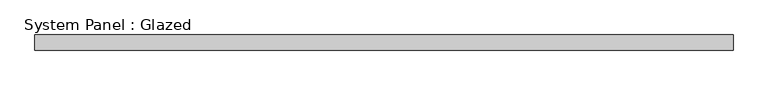
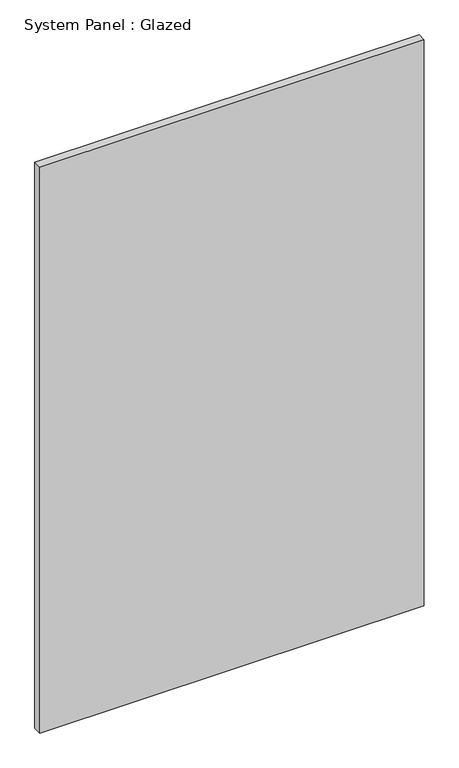
"""IFC4 building model written with IfcOpenShell, lengths in millimetres: plate geometry, System Panel : Glazed."""

from ifc_helpers import new_model, si_unit, origin, origin_with_axes, place, context, project, spatial, polyline, outline, extrude, source, transform, mapped, element, save


def system_panel_glazed_efe6ecb3(model_context):
    return source(origin(), model_context, "Body", "SweptSolid", [
        extrude(outline(polyline([(562.5, 24.5), (-562.5, 24.5), (-562.5, 49.5), (562.5, 49.5), (562.5, 24.5)])), origin_with_axes(), (0.0, 0.0, 1.0), 1750.0),
    ])


if __name__ == "__main__":
    model = new_model("IFC4")
    model_context = context("Model", 3, world=origin())
    ifc_project = project(units=[si_unit("LENGTHUNIT", "METRE", prefix="MILLI")], contexts=[model_context])
    site = spatial("IfcSite", under=ifc_project)
    building = spatial("IfcBuilding", under=site)
    placement = place(None, origin())
    system_panel_glazed_shape = system_panel_glazed_efe6ecb3(model_context)
    element("IfcPlate", 1, ObjectType="System Panel : Glazed", at=placement, inside=building, context=model_context, shape_type="MappedRepresentation", body=[
        mapped(system_panel_glazed_shape, transform((0.0, 0.0, 0.0), x_axis=(1.0, 0.0, 0.0), y_axis=(0.0, 1.0, 0.0), z_axis=(0.0, 0.0, 1.0))),
    ])
    save(model, "model.ifc")

# Revit data of these elements
# Type "System Panel : Glazed"
#   Construction Type Id = "GSP4R"
#   Analytic Construction = "1/8 in Pilkington single glazing"
#   Visual Light Transmittance = 0.9
#   Solar Heat Gain Coefficient = 0.86
#   Heat Transfer Coefficient (U) = 6.7069 W/(m²·K)
#   Define Thermal Properties by = 1
# Element 1 (IfcPlate, "System Panel : Glazed")
#   Materials on its faces: "Glass"
# Materials
#   "Glass": class "Glass", colour RGB 245 245 243, transparency 1, Description = "Soda Lime Glass", Cost = 0
